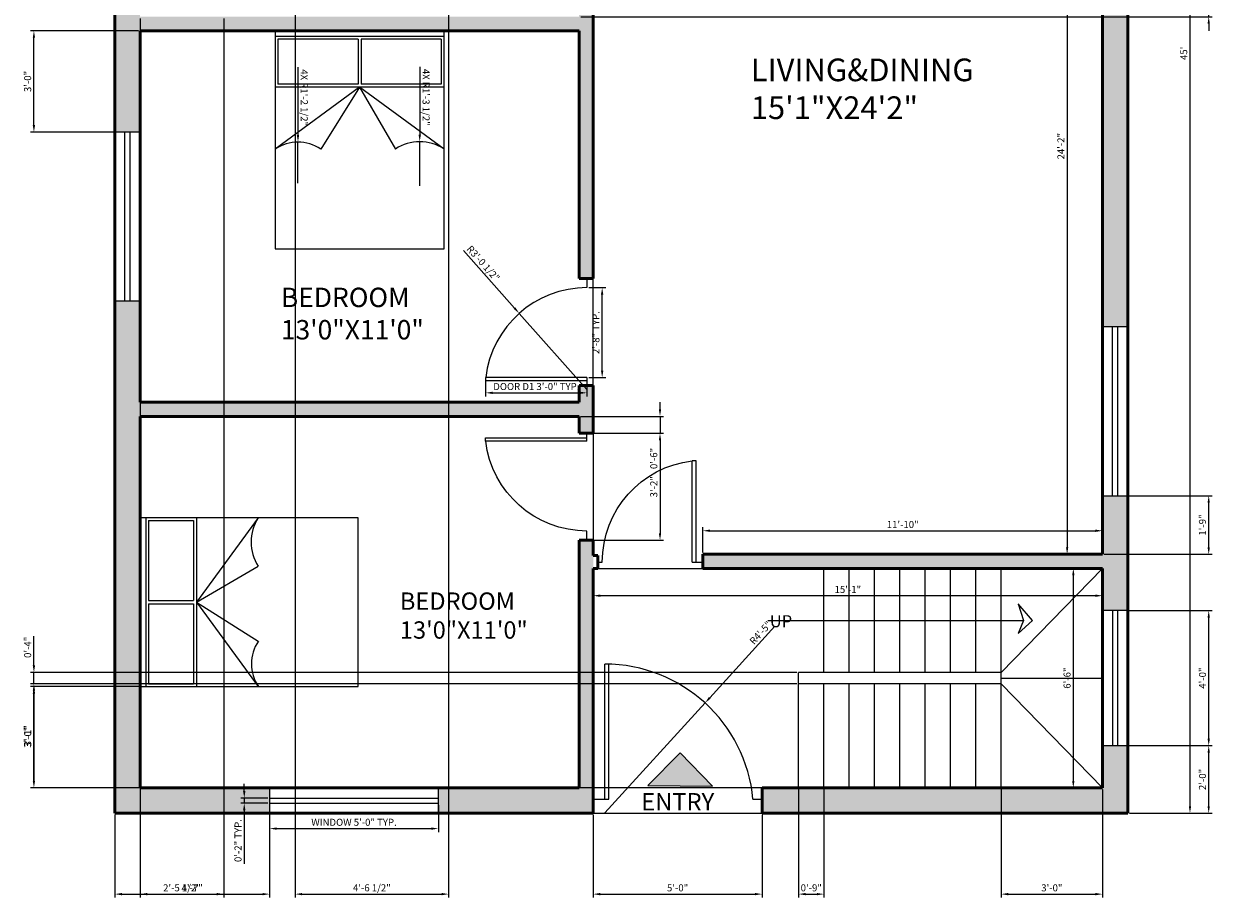
# Model space of a CAD drawing. Units: inches. Extents: x 457 to 882, y 0 to 1111.
# Tile 2 of 4: x 459 to 881, y 506 to 817. Entities that reach past the tile are written whole.
import ezdxf

# ---------------------------------------------------------------- set-up
doc = ezdxf.new("R2010")
doc.units = ezdxf.units.IN
for name, color, linetype, lineweight in [('A-ANNO-DIMS', 2, 'Continuous', 18), ('A-ANNO-SYMB', 7, 'Continuous', 18), ('A-ANNO-SYMB-PATT', 8, 'Continuous', 13), ('A-ANNO-TEXT', 7, 'Continuous', 18), ('A-AREA-IDEN', 7, 'Continuous', 25), ('A-DOOR', 3, 'Continuous', 25), ('A-DOOR-THRE', 8, 'Continuous', 13), ('A-FLOR-STRS', 7, 'Continuous', 25), ('A-FURN', 8, 'Continuous', 18), ('A-GLAZ', 5, 'Continuous', 18), ('A-WALL', 7, 'Continuous', 50), ('A-WALL-PATT', 252, 'Continuous', 13)]:
    doc.layers.add(name, color=color, linetype=linetype, lineweight=lineweight)
doc.styles.get("Standard").update_dxf_attribs({"font": 'arial.ttf'})
doc.dimstyles.new('ISO-25', dxfattribs={"dimtxt": 2.5, "dimasz": 2.5, "dimexe": 1.25, "dimexo": 0.625, "dimtad": 1, "dimdec": 0, "dimlunit": 3, "dimtxsty": 'Standard', "dimcen": 2.5, "dimadec": 0, "dimazin": 0, "dimtfac": 1, "dimtdec": 0, "dimtmove": 0, "dimatfit": 3, "dimfxl": 1, "dimarcsym": 0})

# ---------------------------------------------------------------- blocks, each defined once
blk = doc.blocks.new('*D1')
at = {"layer": 'A-ANNO-DIMS', "color": 0, "lineweight": -2, "transparency": 16777216}
for p, q in [((841.63, 623.51), (830.64, 623.51)), ((831.89, 621.01), (831.89, 548.01)), ((841.63, 545.51), (830.64, 545.51))]:
    blk.add_line(p, q, dxfattribs=at)
at = {"layer": 'A-ANNO-DIMS', "color": 0, "transparency": 16777216}
for points in [[(831.47, 621.01), (832.31, 621.01), (831.89, 623.51)], [(831.47, 548.01), (832.31, 548.01), (831.89, 545.51)]]:
    blk.add_solid(points, dxfattribs=at)
at = {"layer": 'Defpoints', "color": 0, "transparency": 16777216}
for p in [(842.26, 623.51), (831.89, 545.51), (842.26, 545.51)]:
    blk.add_point(p, dxfattribs=at)
at = {"layer": 'A-ANNO-DIMS', "color": 0, "transparency": 16777216, "insert": (829.99, 584.51), "char_height": 2.5, "attachment_point": 5, "rotation": 90}
blk.add_mtext('6\'-6"', dxfattribs=at)
blk = doc.blocks.new('*D3')
at = {"layer": 'A-ANNO-DIMS', "color": 0, "lineweight": -2, "transparency": 16777216}
for p, q in [((851.88, 1076.51), (874.6, 1076.51)), ((873.35, 1074.01), (873.35, 539.01)), ((851.88, 536.51), (874.6, 536.51))]:
    blk.add_line(p, q, dxfattribs=at)
at = {"layer": 'A-ANNO-DIMS', "color": 0, "transparency": 16777216}
for points in [[(872.93, 1074.01), (873.76, 1074.01), (873.35, 1076.51)], [(872.93, 539.01), (873.76, 539.01), (873.35, 536.51)]]:
    blk.add_solid(points, dxfattribs=at)
at = {"layer": 'Defpoints', "color": 0, "transparency": 16777216}
for p in [(851.26, 1076.51), (851.26, 536.51), (873.35, 536.51)]:
    blk.add_point(p, dxfattribs=at)
at = {"layer": 'A-ANNO-DIMS', "color": 0, "transparency": 16777216, "insert": (871.45, 806.51), "char_height": 2.5, "attachment_point": 5, "rotation": 90}
blk.add_mtext("45'", dxfattribs=at)
blk = doc.blocks.new('*D5')
at = {"layer": 'A-ANNO-DIMS', "color": 0, "lineweight": -2, "transparency": 16777216}
for p, q in [((700.26, 629.13), (700.26, 638.12)), ((842.26, 629.13), (842.26, 638.12)), ((702.76, 636.87), (839.76, 636.87))]:
    blk.add_line(p, q, dxfattribs=at)
at = {"layer": 'A-ANNO-DIMS', "color": 0, "transparency": 16777216}
for points in [[(702.76, 637.29), (702.76, 636.46), (700.26, 636.87)], [(839.76, 637.29), (839.76, 636.46), (842.26, 636.87)]]:
    blk.add_solid(points, dxfattribs=at)
at = {"layer": 'Defpoints', "color": 0, "transparency": 16777216}
for p in [(842.26, 636.87), (700.26, 628.51), (842.26, 628.51)]:
    blk.add_point(p, dxfattribs=at)
at = {"layer": 'A-ANNO-DIMS', "color": 0, "transparency": 16777216, "insert": (771.26, 638.77), "char_height": 2.5, "attachment_point": 5}
blk.add_mtext('11\'-10"', dxfattribs=at)
blk = doc.blocks.new('*D7')
at = {"layer": 'A-ANNO-DIMS', "color": 0, "lineweight": -2, "transparency": 16777216}
for p, q in [((841.63, 918.51), (828.45, 918.51)), ((829.7, 916.01), (829.7, 631.01)), ((841.63, 628.51), (828.45, 628.51))]:
    blk.add_line(p, q, dxfattribs=at)
at = {"layer": 'A-ANNO-DIMS', "color": 0, "transparency": 16777216}
for points in [[(829.28, 916.01), (830.11, 916.01), (829.7, 918.51)], [(829.28, 631.01), (830.11, 631.01), (829.7, 628.51)]]:
    blk.add_solid(points, dxfattribs=at)
at = {"layer": 'Defpoints', "color": 0, "transparency": 16777216}
for p in [(842.26, 918.51), (829.7, 628.51), (842.26, 628.51)]:
    blk.add_point(p, dxfattribs=at)
at = {"layer": 'A-ANNO-DIMS', "color": 0, "transparency": 16777216, "insert": (827.82, 773.51), "char_height": 2.5, "attachment_point": 5, "rotation": 90}
blk.add_mtext('24\'-2"', dxfattribs=at)
blk = doc.blocks.new('*D8')
at = {"layer": 'A-ANNO-DIMS', "color": 0, "lineweight": -2, "transparency": 16777216}
for p, q in [((661.26, 622.88), (661.26, 612.55)), ((842.26, 622.88), (842.26, 612.55)), ((839.76, 613.8), (663.76, 613.8))]:
    blk.add_line(p, q, dxfattribs=at)
at = {"layer": 'A-ANNO-DIMS', "color": 0, "transparency": 16777216}
for points in [[(663.76, 614.22), (663.76, 613.38), (661.26, 613.8)], [(839.76, 614.22), (839.76, 613.38), (842.26, 613.8)]]:
    blk.add_solid(points, dxfattribs=at)
at = {"layer": 'Defpoints', "color": 0, "transparency": 16777216}
for p in [(661.26, 623.51), (842.26, 623.51), (661.26, 613.8)]:
    blk.add_point(p, dxfattribs=at)
at = {"layer": 'A-ANNO-DIMS', "color": 0, "transparency": 16777216, "insert": (751.76, 615.7), "char_height": 2.5, "attachment_point": 5}
blk.add_mtext('15\'-1"', dxfattribs=at)
blk = doc.blocks.new('BED-DOUBLE-60')
for p, q in [((0, 77.49), (0, 0)), ((60, 77.49), (0, 77.49)), ((60, 0), (60, 77.49)), ((60, 75.49), (0, 75.49)), ((29.44, 74.49), (0.94, 74.49)), ((0.94, 74.49), (0.94, 58.49)), ((29.44, 74.49), (29.44, 58.49)), ((59, 74.49), (30.53, 74.49)), ((30.53, 74.49), (30.53, 58.49)), ((59, 74.49), (59, 58.49)), ((60, 57.49), (0, 57.49)), ((30, 57.49), (0, 35.49)), ((29.44, 58.49), (0.94, 58.49)), ((30, 57.49), (16.16, 35.49)), ((60, 35.49), (30, 57.49)), ((30, 57.49), (42.73, 35.49)), ((59, 58.49), (30.53, 58.49)), ((0, 0), (60, 0))]:
    blk.add_line(p, q)
for centre, radius, start, end in [((51.36, 22.4), 15.69, 56.5972, 123.4028), ((8.08, 23.34), 14.59, 56.3669, 123.6331)]:
    blk.add_arc(centre, radius, start, end)
blk = doc.blocks.new('WIN-60-GLAZING')
for p, q in [((0, 0), (0, 60)), ((1.86, 0), (1.86, 60))]:
    blk.add_line(p, q)
blk = doc.blocks.new('DOOR-36-SWING')
blk.add_line((36, 0), (0, 0))
blk.add_arc((36, -4.26), 36.25, 90, 173.2534)
blk = doc.blocks.new('*D14')
at = {"layer": 'A-ANNO-DIMS', "color": 0, "lineweight": -2, "transparency": 16777216}
for p, q in [((546.26, 539.41), (546.26, 529.79)), ((606.26, 539.41), (606.26, 529.79)), ((548.76, 531.04), (603.76, 531.04))]:
    blk.add_line(p, q, dxfattribs=at)
at = {"layer": 'A-ANNO-DIMS', "color": 0, "transparency": 16777216}
for points in [[(548.76, 531.45), (548.76, 530.62), (546.26, 531.04)], [(603.76, 531.45), (603.76, 530.62), (606.26, 531.04)]]:
    blk.add_solid(points, dxfattribs=at)
at = {"layer": 'Defpoints', "color": 0, "transparency": 16777216}
for p in [(546.26, 540.04), (606.26, 540.04), (606.26, 531.04)]:
    blk.add_point(p, dxfattribs=at)
at = {"layer": 'A-ANNO-DIMS', "color": 0, "transparency": 16777216, "insert": (576.26, 532.96), "char_height": 2.5, "attachment_point": 5}
blk.add_mtext('WINDOW 5\'-0" TYP.', dxfattribs=at)
blk = doc.blocks.new('*D15')
at = {"layer": 'A-ANNO-DIMS', "color": 0, "lineweight": -2, "transparency": 16777216}
for p, q in [((537.26, 544.4), (537.26, 546.9)), ((545.63, 541.9), (536.01, 541.9)), ((537.26, 541.9), (537.26, 540.04)), ((545.63, 540.04), (536.01, 540.04)), ((537.26, 537.54), (537.26, 518.55))]:
    blk.add_line(p, q, dxfattribs=at)
at = {"layer": 'A-ANNO-DIMS', "color": 0, "transparency": 16777216}
for points in [[(536.84, 544.4), (537.67, 544.4), (537.26, 541.9)], [(536.84, 537.54), (537.67, 537.54), (537.26, 540.04)]]:
    blk.add_solid(points, dxfattribs=at)
at = {"layer": 'Defpoints', "color": 0, "transparency": 16777216}
for p in [(546.26, 541.9), (537.26, 540.04), (546.26, 540.04)]:
    blk.add_point(p, dxfattribs=at)
at = {"layer": 'A-ANNO-DIMS', "color": 0, "transparency": 16777216, "insert": (535.36, 526.79), "char_height": 2.5, "attachment_point": 5, "rotation": 90}
blk.add_mtext('0\'-2" TYP.', dxfattribs=at)
blk = doc.blocks.new('*D18')
at = {"layer": 'A-ANNO-DIMS', "color": 0, "lineweight": -2, "transparency": 16777216}
for p, q in [((623.05, 690.65), (623.05, 684.62)), ((659.05, 690.65), (659.05, 684.62)), ((625.55, 685.87), (656.55, 685.87))]:
    blk.add_line(p, q, dxfattribs=at)
at = {"layer": 'A-ANNO-DIMS', "color": 0, "transparency": 16777216}
for points in [[(625.55, 686.29), (625.55, 685.46), (623.05, 685.87)], [(656.55, 686.29), (656.55, 685.46), (659.05, 685.87)]]:
    blk.add_solid(points, dxfattribs=at)
at = {"layer": 'Defpoints', "color": 0, "transparency": 16777216}
for p in [(623.05, 691.27), (659.05, 691.27), (659.05, 685.87)]:
    blk.add_point(p, dxfattribs=at)
at = {"layer": 'A-ANNO-DIMS', "color": 0, "transparency": 16777216, "insert": (641.05, 687.79), "char_height": 2.5, "attachment_point": 5}
blk.add_mtext('DOOR D1 3\'-0" TYP.', dxfattribs=at)
blk = doc.blocks.new('*D19')
at = {"layer": 'A-ANNO-DIMS', "color": 0, "lineweight": -2, "transparency": 16777216}
for p, q in [((659.68, 723.27), (665.7, 723.27)), ((664.45, 693.77), (664.45, 720.77)), ((659.68, 691.27), (665.7, 691.27))]:
    blk.add_line(p, q, dxfattribs=at)
at = {"layer": 'A-ANNO-DIMS', "color": 0, "transparency": 16777216}
for points in [[(664.03, 720.77), (664.87, 720.77), (664.45, 723.27)], [(664.03, 693.77), (664.87, 693.77), (664.45, 691.27)]]:
    blk.add_solid(points, dxfattribs=at)
at = {"layer": 'Defpoints', "color": 0, "transparency": 16777216}
for p in [(659.05, 723.27), (664.45, 723.27), (659.05, 691.27)]:
    blk.add_point(p, dxfattribs=at)
at = {"layer": 'A-ANNO-DIMS', "color": 0, "transparency": 16777216, "insert": (662.55, 707.27), "char_height": 2.5, "attachment_point": 5, "rotation": 90}
blk.add_mtext('2\'-8" TYP.', dxfattribs=at)
blk = doc.blocks.new('*D25')
at = {"layer": 'A-ANNO-DIMS', "color": 0, "lineweight": -2, "transparency": 16777216}
for p, q in [((656.88, 671.51), (686.26, 671.51)), ((685.01, 669.01), (685.01, 636.01)), ((656.88, 633.51), (686.26, 633.51))]:
    blk.add_line(p, q, dxfattribs=at)
at = {"layer": 'A-ANNO-DIMS', "color": 0, "transparency": 16777216}
for points in [[(684.59, 669.01), (685.42, 669.01), (685.01, 671.51)], [(684.59, 636.01), (685.42, 636.01), (685.01, 633.51)]]:
    blk.add_solid(points, dxfattribs=at)
at = {"layer": 'Defpoints', "color": 0, "transparency": 16777216}
for p in [(656.26, 671.51), (656.26, 633.51), (685.01, 633.51)]:
    blk.add_point(p, dxfattribs=at)
at = {"layer": 'A-ANNO-DIMS', "color": 0, "transparency": 16777216, "insert": (683.11, 652.51), "char_height": 2.5, "attachment_point": 5, "rotation": 90}
blk.add_mtext('3\'-2"', dxfattribs=at)
blk = doc.blocks.new('*D26')
at = {"layer": 'A-ANNO-DIMS', "color": 0, "lineweight": -2, "transparency": 16777216}
for p, q in [((685.01, 680.01), (685.01, 682.51)), ((656.88, 677.51), (686.26, 677.51)), ((685.01, 677.51), (685.01, 671.51)), ((656.88, 671.51), (686.26, 671.51)), ((685.01, 669.01), (685.01, 658.61))]:
    blk.add_line(p, q, dxfattribs=at)
at = {"layer": 'A-ANNO-DIMS', "color": 0, "transparency": 16777216}
for points in [[(684.59, 680.01), (685.42, 680.01), (685.01, 677.51)], [(684.59, 669.01), (685.42, 669.01), (685.01, 671.51)]]:
    blk.add_solid(points, dxfattribs=at)
at = {"layer": 'Defpoints', "color": 0, "transparency": 16777216}
for p in [(656.26, 677.51), (656.26, 671.51), (685.01, 671.51)]:
    blk.add_point(p, dxfattribs=at)
at = {"layer": 'A-ANNO-DIMS', "color": 0, "transparency": 16777216, "insert": (683.11, 662.56), "char_height": 2.5, "attachment_point": 5, "rotation": 90}
blk.add_mtext('0\'-6"', dxfattribs=at)
blk = doc.blocks.new('*D32')
at = {"layer": 'A-ANNO-DIMS', "color": 0, "lineweight": -2, "transparency": 16777216}
for p, q in [((499.63, 814.51), (461.26, 814.51)), ((462.51, 781.01), (462.51, 812.01)), ((490.63, 778.51), (461.26, 778.51))]:
    blk.add_line(p, q, dxfattribs=at)
at = {"layer": 'A-ANNO-DIMS', "color": 0, "transparency": 16777216}
for points in [[(462.09, 812.01), (462.92, 812.01), (462.51, 814.51)], [(462.09, 781.01), (462.92, 781.01), (462.51, 778.51)]]:
    blk.add_solid(points, dxfattribs=at)
at = {"layer": 'Defpoints', "color": 0, "transparency": 16777216}
for p in [(462.51, 814.51), (500.26, 814.51), (491.26, 778.51)]:
    blk.add_point(p, dxfattribs=at)
at = {"layer": 'A-ANNO-DIMS', "color": 0, "transparency": 16777216, "insert": (460.61, 796.51), "char_height": 2.5, "attachment_point": 5, "rotation": 90}
blk.add_mtext('3\'-0"', dxfattribs=at)
blk = doc.blocks.new('*D33')
at = {"layer": 'A-ANNO-DIMS', "color": 0, "lineweight": -2, "transparency": 16777216}
for p, q in [((491.26, 535.88), (491.26, 506.51)), ((546.26, 535.88), (546.26, 506.51)), ((493.76, 507.76), (543.76, 507.76))]:
    blk.add_line(p, q, dxfattribs=at)
at = {"layer": 'A-ANNO-DIMS', "color": 0, "transparency": 16777216}
for points in [[(493.76, 508.17), (493.76, 507.34), (491.26, 507.76)], [(543.76, 508.17), (543.76, 507.34), (546.26, 507.76)]]:
    blk.add_solid(points, dxfattribs=at)
at = {"layer": 'Defpoints', "color": 0, "transparency": 16777216}
for p in [(491.26, 536.51), (546.26, 536.51), (546.26, 507.76)]:
    blk.add_point(p, dxfattribs=at)
at = {"layer": 'A-ANNO-DIMS', "color": 0, "transparency": 16777216, "insert": (518.76, 509.63), "char_height": 2.5, "attachment_point": 5}
blk.add_mtext('4\'-7"', dxfattribs=at)
blk = doc.blocks.new('*D35')
at = {"layer": 'A-ANNO-DIMS', "color": 0, "lineweight": -2, "transparency": 16777216}
for p, q in [((851.88, 649.3), (881.26, 649.3)), ((880.01, 631.01), (880.01, 646.8)), ((842.88, 628.51), (881.26, 628.51))]:
    blk.add_line(p, q, dxfattribs=at)
at = {"layer": 'A-ANNO-DIMS', "color": 0, "transparency": 16777216}
for points in [[(879.59, 646.8), (880.42, 646.8), (880.01, 649.3)], [(879.59, 631.01), (880.42, 631.01), (880.01, 628.51)]]:
    blk.add_solid(points, dxfattribs=at)
at = {"layer": 'Defpoints', "color": 0, "transparency": 16777216}
for p in [(851.26, 649.3), (880.01, 649.3), (842.26, 628.51)]:
    blk.add_point(p, dxfattribs=at)
at = {"layer": 'A-ANNO-DIMS', "color": 0, "transparency": 16777216, "insert": (878.11, 638.9), "char_height": 2.5, "attachment_point": 5, "rotation": 90}
blk.add_mtext('1\'-9"', dxfattribs=at)
blk = doc.blocks.new('*D38')
at = {"layer": 'A-ANNO-DIMS', "color": 0, "lineweight": -2, "transparency": 16777216}
for p, q in [((851.88, 608.51), (881.26, 608.51)), ((880.01, 563.01), (880.01, 606.01)), ((851.88, 560.51), (881.26, 560.51))]:
    blk.add_line(p, q, dxfattribs=at)
at = {"layer": 'A-ANNO-DIMS', "color": 0, "transparency": 16777216}
for points in [[(879.59, 606.01), (880.42, 606.01), (880.01, 608.51)], [(879.59, 563.01), (880.42, 563.01), (880.01, 560.51)]]:
    blk.add_solid(points, dxfattribs=at)
at = {"layer": 'Defpoints', "color": 0, "transparency": 16777216}
for p in [(851.26, 608.51), (880.01, 608.51), (851.26, 560.51)]:
    blk.add_point(p, dxfattribs=at)
at = {"layer": 'A-ANNO-DIMS', "color": 0, "transparency": 16777216, "insert": (878.11, 584.51), "char_height": 2.5, "attachment_point": 5, "rotation": 90}
blk.add_mtext('4\'-0"', dxfattribs=at)
blk = doc.blocks.new('*D39')
at = {"layer": 'A-ANNO-DIMS', "color": 0, "lineweight": -2, "transparency": 16777216}
for p, q in [((851.88, 560.51), (881.26, 560.51)), ((880.01, 539.01), (880.01, 558.01)), ((851.88, 536.51), (881.26, 536.51))]:
    blk.add_line(p, q, dxfattribs=at)
at = {"layer": 'A-ANNO-DIMS', "color": 0, "transparency": 16777216}
for points in [[(879.59, 558.01), (880.42, 558.01), (880.01, 560.51)], [(879.59, 539.01), (880.42, 539.01), (880.01, 536.51)]]:
    blk.add_solid(points, dxfattribs=at)
at = {"layer": 'Defpoints', "color": 0, "transparency": 16777216}
for p in [(851.26, 560.51), (880.01, 560.51), (851.26, 536.51)]:
    blk.add_point(p, dxfattribs=at)
at = {"layer": 'A-ANNO-DIMS', "color": 0, "transparency": 16777216, "insert": (878.11, 548.51), "char_height": 2.5, "attachment_point": 5, "rotation": 90}
blk.add_mtext('2\'-0"', dxfattribs=at)
blk = doc.blocks.new('*D40')
at = {"layer": 'A-ANNO-DIMS', "color": 0, "lineweight": -2, "transparency": 16777216}
for p, q in [((661.26, 535.88), (661.26, 506.51)), ((721.26, 535.88), (721.26, 506.51)), ((663.76, 507.76), (718.76, 507.76))]:
    blk.add_line(p, q, dxfattribs=at)
at = {"layer": 'A-ANNO-DIMS', "color": 0, "transparency": 16777216}
for points in [[(663.76, 508.17), (663.76, 507.34), (661.26, 507.76)], [(718.76, 508.17), (718.76, 507.34), (721.26, 507.76)]]:
    blk.add_solid(points, dxfattribs=at)
at = {"layer": 'Defpoints', "color": 0, "transparency": 16777216}
for p in [(661.26, 536.51), (721.26, 536.51), (721.26, 507.76)]:
    blk.add_point(p, dxfattribs=at)
at = {"layer": 'A-ANNO-DIMS', "color": 0, "transparency": 16777216, "insert": (691.26, 509.66), "char_height": 2.5, "attachment_point": 5}
blk.add_mtext('5\'-0"', dxfattribs=at)
blk = doc.blocks.new('*D41')
at = {"layer": 'A-ANNO-DIMS', "color": 0, "lineweight": -2, "transparency": 16777216}
for p, q in [((734.26, 544.88), (734.26, 506.51)), ((743.26, 544.88), (743.26, 506.51)), ((736.76, 507.76), (740.76, 507.76))]:
    blk.add_line(p, q, dxfattribs=at)
at = {"layer": 'A-ANNO-DIMS', "color": 0, "transparency": 16777216}
for points in [[(736.76, 508.17), (736.76, 507.34), (734.26, 507.76)], [(740.76, 508.17), (740.76, 507.34), (743.26, 507.76)]]:
    blk.add_solid(points, dxfattribs=at)
at = {"layer": 'Defpoints', "color": 0, "transparency": 16777216}
for p in [(734.26, 545.51), (743.26, 545.51), (743.26, 507.76)]:
    blk.add_point(p, dxfattribs=at)
at = {"layer": 'A-ANNO-DIMS', "color": 0, "transparency": 16777216, "insert": (738.76, 509.66), "char_height": 2.5, "attachment_point": 5}
blk.add_mtext('0\'-9"', dxfattribs=at)
blk = doc.blocks.new('*D42')
at = {"layer": 'A-ANNO-DIMS', "color": 0, "lineweight": -2, "transparency": 16777216}
for p, q in [((806.26, 544.88), (806.26, 506.51)), ((842.26, 544.88), (842.26, 506.51)), ((808.76, 507.76), (839.76, 507.76))]:
    blk.add_line(p, q, dxfattribs=at)
at = {"layer": 'A-ANNO-DIMS', "color": 0, "transparency": 16777216}
for points in [[(808.76, 508.17), (808.76, 507.34), (806.26, 507.76)], [(839.76, 508.17), (839.76, 507.34), (842.26, 507.76)]]:
    blk.add_solid(points, dxfattribs=at)
at = {"layer": 'Defpoints', "color": 0, "transparency": 16777216}
for p in [(806.26, 545.51), (842.26, 545.51), (842.26, 507.76)]:
    blk.add_point(p, dxfattribs=at)
at = {"layer": 'A-ANNO-DIMS', "color": 0, "transparency": 16777216, "insert": (824.26, 509.66), "char_height": 2.5, "attachment_point": 5}
blk.add_mtext('3\'-0"', dxfattribs=at)
blk = doc.blocks.new('*D43')
at = {"layer": 'A-ANNO-DIMS', "color": 0, "lineweight": -2, "transparency": 16777216}
for p, q in [((733.63, 582.51), (461.26, 582.51)), ((462.51, 548.01), (462.51, 580.01)), ((733.63, 545.51), (461.26, 545.51))]:
    blk.add_line(p, q, dxfattribs=at)
at = {"layer": 'A-ANNO-DIMS', "color": 0, "transparency": 16777216}
for points in [[(462.09, 580.01), (462.92, 580.01), (462.51, 582.51)], [(462.09, 548.01), (462.92, 548.01), (462.51, 545.51)]]:
    blk.add_solid(points, dxfattribs=at)
at = {"layer": 'Defpoints', "color": 0, "transparency": 16777216}
for p in [(462.51, 582.51), (734.26, 582.51), (734.26, 545.51)]:
    blk.add_point(p, dxfattribs=at)
at = {"layer": 'A-ANNO-DIMS', "color": 0, "transparency": 16777216, "insert": (460.61, 564.01), "char_height": 2.5, "attachment_point": 5, "rotation": 90}
blk.add_mtext('3\'-1"', dxfattribs=at)
blk = doc.blocks.new('*D44')
at = {"layer": 'A-ANNO-DIMS', "color": 0, "lineweight": -2, "transparency": 16777216}
for p, q in [((462.51, 589.01), (462.51, 599.4)), ((733.63, 586.51), (461.26, 586.51)), ((462.51, 582.51), (462.51, 586.51)), ((733.63, 582.51), (461.26, 582.51)), ((462.51, 580.01), (462.51, 577.51))]:
    blk.add_line(p, q, dxfattribs=at)
at = {"layer": 'A-ANNO-DIMS', "color": 0, "transparency": 16777216}
for points in [[(462.09, 589.01), (462.92, 589.01), (462.51, 586.51)], [(462.09, 580.01), (462.92, 580.01), (462.51, 582.51)]]:
    blk.add_solid(points, dxfattribs=at)
at = {"layer": 'Defpoints', "color": 0, "transparency": 16777216}
for p in [(462.51, 586.51), (734.26, 586.51), (734.26, 582.51)]:
    blk.add_point(p, dxfattribs=at)
at = {"layer": 'A-ANNO-DIMS', "color": 0, "transparency": 16777216, "insert": (460.61, 595.45), "char_height": 2.5, "attachment_point": 5, "rotation": 90}
blk.add_mtext('0\'-4"', dxfattribs=at)
blk = doc.blocks.new('*D45')
at = {"layer": 'A-ANNO-DIMS', "color": 0, "lineweight": -2, "transparency": 16777216}
for p, q in [((500.26, 818.88), (500.26, 506.51)), ((530, 818.88), (530, 506.51)), ((502.76, 507.76), (527.5, 507.76))]:
    blk.add_line(p, q, dxfattribs=at)
at = {"layer": 'A-ANNO-DIMS', "color": 0, "transparency": 16777216}
for points in [[(502.76, 508.17), (502.76, 507.34), (500.26, 507.76)], [(527.5, 508.17), (527.5, 507.34), (530, 507.76)]]:
    blk.add_solid(points, dxfattribs=at)
at = {"layer": 'Defpoints', "color": 0, "transparency": 16777216}
for p in [(500.26, 819.51), (530, 819.51), (530, 507.76)]:
    blk.add_point(p, dxfattribs=at)
at = {"layer": 'A-ANNO-DIMS', "color": 0, "transparency": 16777216, "insert": (515.13, 509.67), "char_height": 2.5, "attachment_point": 5}
blk.add_mtext('2\'-5 1/2"', dxfattribs=at)
blk = doc.blocks.new('*D48')
at = {"layer": 'A-ANNO-DIMS', "color": 0, "lineweight": -2, "transparency": 16777216}
for p, q in [((880.01, 828.01), (880.01, 838.4)), ((656.88, 825.51), (881.26, 825.51)), ((880.01, 819.51), (880.01, 825.51)), ((656.88, 819.51), (881.26, 819.51)), ((880.01, 817.01), (880.01, 814.51))]:
    blk.add_line(p, q, dxfattribs=at)
at = {"layer": 'A-ANNO-DIMS', "color": 0, "transparency": 16777216}
for points in [[(879.59, 828.01), (880.42, 828.01), (880.01, 825.51)], [(879.59, 817.01), (880.42, 817.01), (880.01, 819.51)]]:
    blk.add_solid(points, dxfattribs=at)
at = {"layer": 'Defpoints', "color": 0, "transparency": 16777216}
for p in [(656.26, 825.51), (880.01, 825.51), (656.26, 819.51)]:
    blk.add_point(p, dxfattribs=at)
at = {"layer": 'A-ANNO-DIMS', "color": 0, "transparency": 16777216, "insert": (878.11, 834.45), "char_height": 2.5, "attachment_point": 5, "rotation": 90}
blk.add_mtext('0\'-6"', dxfattribs=at)
blk = doc.blocks.new('*D56')
at = {"layer": 'A-ANNO-DIMS', "color": 0, "lineweight": -2, "transparency": 16777216}
for p, q in [((555.33, 898.14), (555.33, 506.51)), ((609.9, 898.14), (609.9, 506.51)), ((557.83, 507.76), (607.4, 507.76))]:
    blk.add_line(p, q, dxfattribs=at)
at = {"layer": 'A-ANNO-DIMS', "color": 0, "transparency": 16777216}
for points in [[(557.83, 508.17), (557.83, 507.34), (555.33, 507.76)], [(607.4, 508.17), (607.4, 507.34), (609.9, 507.76)]]:
    blk.add_solid(points, dxfattribs=at)
at = {"layer": 'Defpoints', "color": 0, "transparency": 16777216}
for p in [(555.33, 898.77), (609.9, 898.77), (609.9, 507.76)]:
    blk.add_point(p, dxfattribs=at)
at = {"layer": 'A-ANNO-DIMS', "color": 0, "transparency": 16777216, "insert": (582.61, 509.67), "char_height": 2.5, "attachment_point": 5}
blk.add_mtext('4\'-6 1/2"', dxfattribs=at)
blk = doc.blocks.new('*D60')
at = {"layer": 'A-ANNO-DIMS', "color": 0, "lineweight": -2, "transparency": 16777216}
for p, q in [((499.63, 581.51), (461.26, 581.51)), ((462.51, 579.01), (462.51, 548.01)), ((499.63, 545.51), (461.26, 545.51))]:
    blk.add_line(p, q, dxfattribs=at)
at = {"layer": 'A-ANNO-DIMS', "color": 0, "transparency": 16777216}
for points in [[(462.09, 579.01), (462.92, 579.01), (462.51, 581.51)], [(462.09, 548.01), (462.92, 548.01), (462.51, 545.51)]]:
    blk.add_solid(points, dxfattribs=at)
at = {"layer": 'Defpoints', "color": 0, "transparency": 16777216}
for p in [(500.26, 581.51), (462.51, 545.51), (500.26, 545.51)]:
    blk.add_point(p, dxfattribs=at)
at = {"layer": 'A-ANNO-DIMS', "color": 0, "transparency": 16777216, "insert": (460.61, 563.51), "char_height": 2.5, "attachment_point": 5, "rotation": 90}
blk.add_mtext('3\'-0"', dxfattribs=at)
blk = doc.blocks.new('*D61')
at = {"layer": 'A-ANNO-DIMS', "color": 0, "lineweight": -2, "transparency": 16777216}
for p, q in [((725.86, 602.94), (702.7, 577.53)), ((665.39, 536.59), (701.01, 575.68))]:
    blk.add_line(p, q, dxfattribs=at)
at = {"layer": 'A-ANNO-DIMS', "color": 0, "transparency": 16777216}
blk.add_solid([(702.39, 577.81), (703.01, 577.25), (701.01, 575.68)], dxfattribs=at)
at = {"layer": 'Defpoints', "color": 0, "transparency": 16777216}
for p in [(701.01, 575.68), (665.39, 536.59)]:
    blk.add_point(p, dxfattribs=at)
at = {"layer": 'A-ANNO-DIMS', "color": 0, "transparency": 16777216, "insert": (720.99, 600.41), "char_height": 2.5, "attachment_point": 5, "rotation": 47.6519}
blk.add_mtext('R4\'-5"', dxfattribs=at)
blk = doc.blocks.new('*D68')
at = {"layer": 'A-ANNO-DIMS', "color": 0, "lineweight": -2, "transparency": 16777216}
for p, q in [((615.17, 736.39), (633.31, 715.98)), ((659.05, 687.01), (634.97, 714.11))]:
    blk.add_line(p, q, dxfattribs=at)
at = {"layer": 'A-ANNO-DIMS', "color": 0, "transparency": 16777216}
blk.add_solid([(633.62, 716.26), (633, 715.7), (634.97, 714.11)], dxfattribs=at)
at = {"layer": 'Defpoints', "color": 0, "transparency": 16777216}
for p in [(634.97, 714.11), (659.05, 687.01)]:
    blk.add_point(p, dxfattribs=at)
at = {"layer": 'A-ANNO-DIMS', "color": 0, "transparency": 16777216, "insert": (621.96, 731.64), "char_height": 2.5, "attachment_point": 5, "rotation": 311.6258}
blk.add_mtext('R3\'-0 1/2"', dxfattribs=at)
blk = doc.blocks.new('*D69')
at = {"layer": 'A-ANNO-DIMS', "color": 0, "lineweight": -2, "transparency": 16777216}
for p, q in [((599.62, 801.68), (599.62, 777.6)), ((599.62, 759.41), (599.62, 775.1))]:
    blk.add_line(p, q, dxfattribs=at)
at = {"layer": 'A-ANNO-DIMS', "color": 0, "transparency": 16777216}
blk.add_solid([(600.04, 777.6), (599.2, 777.6), (599.62, 775.1)], dxfattribs=at)
at = {"layer": 'Defpoints', "color": 0, "transparency": 16777216}
for p in [(599.62, 775.1), (599.62, 759.41)]:
    blk.add_point(p, dxfattribs=at)
at = {"layer": 'A-ANNO-DIMS', "color": 0, "transparency": 16777216, "insert": (601.54, 790.89), "char_height": 2.5, "attachment_point": 5, "rotation": 270.0015}
blk.add_mtext('4X R1\'-3 1/2"', dxfattribs=at)
blk = doc.blocks.new('*D70')
at = {"layer": 'A-ANNO-DIMS', "color": 0, "lineweight": -2, "transparency": 16777216}
for p, q in [((556.34, 801.53), (556.34, 777.45)), ((556.34, 760.35), (556.34, 774.95))]:
    blk.add_line(p, q, dxfattribs=at)
at = {"layer": 'A-ANNO-DIMS', "color": 0, "transparency": 16777216}
blk.add_solid([(556.76, 777.45), (555.92, 777.45), (556.34, 774.95)], dxfattribs=at)
at = {"layer": 'Defpoints', "color": 0, "transparency": 16777216}
for p in [(556.34, 774.95), (556.34, 760.35)]:
    blk.add_point(p, dxfattribs=at)
at = {"layer": 'A-ANNO-DIMS', "color": 0, "transparency": 16777216, "insert": (558.26, 790.74), "char_height": 2.5, "attachment_point": 5, "rotation": 270.001}
blk.add_mtext('4X R1\'-2 1/2"', dxfattribs=at)

msp = doc.modelspace()

# ---------------------------------------------------------------- hatches: boundary and pattern name
at = {"layer": 'A-ANNO-SYMB-PATT'}
h = msp.add_hatch(color=256, dxfattribs=at)
h.dxf.hatch_style = 1
h.paths.add_polyline_path([(692.14, 557.94), (680.67, 546.33), (703.61, 546.11)])
at = {"layer": 'A-WALL-PATT'}
h = msp.add_hatch(color=256, dxfattribs=at)
h.dxf.hatch_style = 1
h.paths.add_polyline_path([(677.26, 1076.51), (491.26, 1076.51), (491.26, 1031.73), (500.26, 1031.73), (500.26, 1067.51), (656.26, 1067.51), (656.26, 962.63), (661.26, 962.63), (661.26, 1067.51), (677.26, 1067.51)])
h.paths.add_polyline_path([(851.26, 1076.51), (701.26, 1076.51), (701.26, 1067.51), (717.26, 1067.51), (717.26, 971.51), (691.26, 971.51), (691.26, 966.51), (717.26, 966.51), (717.26, 962.63), (722.26, 962.63), (722.26, 1067.51), (842.26, 1067.51), (842.26, 1031.73), (851.26, 1031.73)])
h.paths.add_polyline_path([(851.26, 971.73), (842.26, 971.73), (842.26, 923.51), (722.26, 923.51), (722.26, 926.63), (717.26, 926.63), (717.26, 918.51), (842.26, 918.51), (842.26, 896.98), (851.26, 896.98)])
h.paths.add_polyline_path([(661.26, 926.63), (656.26, 926.63), (656.26, 923.51), (500.26, 923.51), (500.26, 971.73), (491.26, 971.73), (491.26, 899.01), (500.26, 899.01), (500.26, 918.51), (656.26, 918.51), (656.26, 873.51), (661.26, 873.51)])
h.paths.add_polyline_path([(500.26, 839.01), (491.26, 839.01), (491.26, 778.51), (500.26, 778.51), (500.26, 814.51), (656.26, 814.51), (656.26, 726.51), (661.26, 726.51), (661.26, 825.51), (656.26, 825.51), (656.26, 819.51), (500.26, 819.51)])
h.paths.add_polyline_path([(661.26, 633.51), (656.26, 633.51), (656.26, 545.51), (606.26, 545.51), (606.26, 536.51), (661.26, 536.51)], flags=0)
h.paths.add_polyline_path([(851.26, 560.51), (842.26, 560.51), (842.26, 545.51), (721.26, 545.51), (721.26, 536.51), (851.26, 536.51)])
h.paths.add_polyline_path([(851.26, 649.3), (842.26, 649.3), (842.26, 628.51), (700.26, 628.51), (700.26, 623.51), (842.26, 623.51), (842.26, 608.51), (851.26, 608.51)])
h.paths.add_polyline_path([(500.26, 677.51), (656.26, 677.51), (656.26, 671.51), (661.26, 671.51), (661.26, 688.51), (656.26, 688.51), (656.26, 682.51), (500.26, 682.51), (500.26, 718.51), (491.26, 718.51), (491.26, 536.51), (546.26, 536.51), (546.26, 545.51), (500.26, 545.51)])
h = msp.add_hatch(color=256, dxfattribs=at)
h.dxf.hatch_style = 1
h.paths.add_polyline_path([(851.26, 836.98), (842.26, 836.98), (842.26, 709.3), (851.26, 709.3)])
h = msp.add_hatch(color=256, dxfattribs=at)
h.dxf.hatch_style = 1
h.paths.add_polyline_path([(661.26, 633.51), (656.26, 633.51), (656.26, 545.51), (606.26, 545.51), (606.26, 536.51), (661.26, 536.51)])

# ---------------------------------------------------------------- linework, layer by layer
at = {"layer": 'A-ANNO-SYMB'}
for p, q in [((817.38, 605.01), (812.27, 610.9)), ((812.27, 610.9), (814.15, 605.01)), ((723.36, 605.01), (814.15, 605.01)), ((812.27, 600.4), (817.38, 605.01)), ((814.15, 605.01), (812.27, 600.4)), ((692.14, 557.94), (680.67, 546.33)), ((703.61, 546.11), (692.14, 557.94)), ((680.67, 546.33), (703.61, 546.11))]:
    msp.add_line(p, q, dxfattribs=at)
at = {"layer": 'A-DOOR'}
for p, q in [((659.05, 726.51), (659.05, 723.27)), ((623.05, 691.27), (623.05, 690.24)), ((623.05, 690.24), (659.05, 690.24)), ((659.05, 691.27), (659.05, 688.51)), ((623.05, 668.74), (623.05, 669.86)), ((623.05, 669.86), (659.05, 669.86)), ((659.05, 668.74), (659.05, 671.51)), ((697.87, 661.73), (696.49, 661.73)), ((697.87, 625.73), (697.87, 661.73)), ((659.05, 633.51), (659.05, 636.74)), ((662.88, 625.73), (664.5, 625.73)), ((696.49, 625.73), (700.26, 625.73)), ((665.39, 541.48), (665.39, 589.48)), ((666.88, 541.48), (666.88, 589.48)), ((661.26, 541.48), (666.88, 541.48)), ((718.05, 541.48), (721.26, 541.48))]:
    msp.add_line(p, q, dxfattribs=at)
msp.add_arc((665.39, 536.59), 52.89, 5.3049, 90, dxfattribs=at)
at = {"layer": 'A-DOOR-THRE'}
for p, q in [((661.26, 688.51), (661.26, 726.51)), ((661.26, 671.51), (661.26, 633.51)), ((662.88, 623.51), (700.26, 623.51)), ((661.26, 536.51), (721.26, 536.51))]:
    msp.add_line(p, q, dxfattribs=at)
at = {"layer": 'A-FLOR-STRS'}
for p, q in [((743.26, 586.51), (743.26, 623.51)), ((752.26, 586.51), (752.26, 623.51)), ((761.26, 586.51), (761.26, 623.51)), ((770.26, 586.51), (770.26, 623.51)), ((779.26, 586.51), (779.26, 623.51)), ((788.26, 586.51), (788.26, 623.51)), ((797.26, 586.51), (797.26, 623.51)), ((806.26, 545.51), (806.26, 623.51)), ((806.26, 586.51), (842.26, 623.51)), ((806.26, 586.51), (734.26, 586.51)), ((734.26, 545.51), (734.26, 586.51)), ((806.26, 584.51), (842.26, 584.51)), ((806.26, 582.51), (734.26, 582.51)), ((743.26, 545.51), (743.26, 582.51)), ((752.26, 545.51), (752.26, 582.51)), ((761.26, 545.51), (761.26, 582.51)), ((770.26, 545.51), (770.26, 582.51)), ((779.26, 545.51), (779.26, 582.51)), ((788.26, 545.51), (788.26, 582.51)), ((797.26, 545.51), (797.26, 582.51)), ((806.26, 582.51), (842.26, 545.51))]:
    msp.add_line(p, q, dxfattribs=at)
at = {"layer": 'A-GLAZ'}
for p, q in [((500.26, 778.51), (491.26, 778.51)), ((491.26, 718.51), (500.26, 718.51)), ((851.26, 709.3), (842.26, 709.3)), ((842.26, 649.3), (851.26, 649.3)), ((851.26, 608.51), (842.26, 608.51)), ((845.79, 608.51), (845.79, 560.51)), ((847.65, 608.51), (847.65, 560.51)), ((842.26, 560.51), (851.26, 560.51)), ((546.26, 545.51), (546.26, 536.51)), ((606.26, 536.51), (606.26, 545.51))]:
    msp.add_line(p, q, dxfattribs=at)
at = {"layer": 'A-WALL'}
for p, q in [((491.26, 1076.51), (491.26, 536.51)), ((851.26, 536.51), (851.26, 1076.51)), ((842.26, 628.51), (842.26, 918.51)), ((661.26, 825.51), (661.26, 726.51)), ((500.26, 814.51), (656.26, 814.51)), ((500.26, 814.51), (500.26, 682.51)), ((656.26, 814.51), (656.26, 726.51)), ((661.26, 726.51), (656.26, 726.51)), ((661.26, 688.51), (656.26, 688.51)), ((656.26, 688.51), (656.26, 682.51)), ((661.26, 688.51), (661.26, 671.51)), ((500.26, 682.51), (656.26, 682.51)), ((500.26, 677.51), (656.26, 677.51)), ((500.26, 677.51), (500.26, 545.51)), ((656.26, 677.51), (656.26, 671.51)), ((661.26, 671.51), (656.26, 671.51)), ((661.26, 633.51), (656.26, 633.51)), ((656.26, 633.51), (656.26, 545.51)), ((661.26, 633.51), (661.26, 628.11)), ((662.88, 628.11), (661.26, 628.11)), ((662.88, 623.51), (662.88, 628.11)), ((662.88, 625.73), (662.88, 623.51)), ((700.26, 623.51), (700.26, 628.51)), ((700.26, 628.51), (842.26, 628.51)), ((662.88, 623.51), (661.26, 623.51)), ((661.26, 623.51), (661.26, 536.51)), ((700.26, 623.51), (842.26, 623.51)), ((842.26, 545.51), (842.26, 623.51)), ((500.26, 545.51), (656.26, 545.51)), ((721.26, 536.51), (721.26, 545.51)), ((721.26, 545.51), (842.26, 545.51)), ((491.26, 536.51), (661.26, 536.51)), ((721.26, 536.51), (851.26, 536.51))]:
    msp.add_line(p, q, dxfattribs=at)

# ---------------------------------------------------------------- block references
at = {"layer": 'A-DOOR'}
msp.add_blockref('DOOR-36-SWING', (623.05, 691.27), dxfattribs=at)
at = {"layer": 'A-DOOR', "extrusion": (0, 0, -1), "zscale": -1}
for p, rotation in [((-623.05, 668.74), 180), ((-696.49, 661.73), 269.9999999999999)]:
    msp.add_blockref('DOOR-36-SWING', p, dxfattribs=dict(at, rotation=rotation))
at = {"layer": 'A-FURN'}
msp.add_blockref('BED-DOUBLE-60', (548.26, 737.01), dxfattribs=at)
at = {"layer": 'A-FURN', "rotation": 90}
msp.add_blockref('BED-DOUBLE-60', (577.75, 581.51), dxfattribs=at)
at = {"layer": 'A-GLAZ'}
for p in [(494.86, 718.5), (845.86, 649.3)]:
    msp.add_blockref('WIN-60-GLAZING', p, dxfattribs=at)
at = {"layer": 'A-GLAZ', "rotation": 270.0000000000001}
msp.add_blockref('WIN-60-GLAZING', (546.26, 541.9), dxfattribs=at)

# ---------------------------------------------------------------- texts
at = {"layer": 'A-ANNO-TEXT', "attachment_point": 1}
for s, width, gutter_width, insert, char_height in [('UP', 56.9254, 21.47, (724.03, 606.87), 4.294), ('ENTRY', 81.9788, 30.92, (678.32, 543.67), 6.184)]:
    msp.add_mtext_dynamic_manual_height_columns(s, width=width, gutter_width=gutter_width, heights=[0], dxfattribs=dict(at, insert=insert, char_height=char_height))
at = {"layer": 'A-AREA-IDEN', "attachment_point": 1}
for s, width, gutter_width, insert, char_height in [('LIVING&DINING\\P15\'1"X24\'2"', 140.6069, 40.29, (717.27, 804.65), 8.058), ('BEDROOM\\P13\'0"X11\'0"', 91.3786, 34.46, (550.26, 723.23), 6.8929), ('BEDROOM\\P13\'0"X11\'0"', 78.4895, 30.8, (592.56, 614.95), 6.1598)]:
    msp.add_mtext_dynamic_manual_height_columns(s, width=width, gutter_width=gutter_width, heights=[0], dxfattribs=dict(at, insert=insert, char_height=char_height))

# ---------------------------------------------------------------- dimensions: what is measured, and where the dimension line sits
at = {"layer": 'A-ANNO-DIMS'}
for base, p1, p2, angle, override, picture, middle in [((873.35, 536.51), (851.26, 1076.51), (851.26, 536.51), 90, {"dimclrd": 0, "dimclre": 0, "dimclrt": 0}, '*D3', (871.45, 806.51)), ((829.7, 628.51), (842.26, 918.51), (842.26, 628.51), 90, {"dimclrd": 0, "dimclre": 0, "dimclrt": 0}, '*D7', (827.82, 773.51)), ((880.01, 825.51), (656.26, 819.51), (656.26, 825.51), 90, {"dimdec": 1, "dimlfac": 1, "dimrnd": 0, "dimzin": 1, "dimdsep": 46, "dimlunit": 4, "dimfrac": 2}, '*D48', (878.11, 834.45)), ((462.51, 814.51), (491.26, 778.51), (500.26, 814.51), 90, {"dimdec": 1, "dimlfac": 1, "dimrnd": 0, "dimzin": 1, "dimdsep": 46, "dimlunit": 4, "dimfrac": 2}, '*D32', (460.61, 796.51)), ((685.01, 671.51), (656.26, 677.51), (656.26, 671.51), 270, {"dimdec": 1, "dimlfac": 1, "dimrnd": 0, "dimzin": 1, "dimdsep": 46, "dimlunit": 4, "dimfrac": 2}, '*D26', (683.11, 662.56)), ((685.01, 633.51), (656.26, 671.51), (656.26, 633.51), 270, {"dimdec": 1, "dimlfac": 1, "dimrnd": 0, "dimzin": 1, "dimdsep": 46, "dimlunit": 4, "dimfrac": 2}, '*D25', (683.11, 652.51)), ((880.01, 649.3), (842.26, 628.51), (851.26, 649.3), 90, {"dimdec": 1, "dimlfac": 1, "dimrnd": 0, "dimzin": 1, "dimdsep": 46, "dimlunit": 4, "dimfrac": 2}, '*D35', (878.11, 638.9)), ((831.89, 545.51), (842.26, 623.51), (842.26, 545.51), 90, {"dimclrd": 0, "dimclre": 0, "dimclrt": 0}, '*D1', (829.99, 584.51)), ((880.01, 608.51), (851.26, 560.51), (851.26, 608.51), 90, {"dimdec": 1, "dimlfac": 1, "dimrnd": 0, "dimzin": 1, "dimdsep": 46, "dimlunit": 4, "dimfrac": 2}, '*D38', (878.11, 584.51)), ((462.51, 586.51), (734.26, 582.51), (734.26, 586.51), 90, {"dimdec": 1, "dimlfac": 1, "dimrnd": 0, "dimzin": 1, "dimdsep": 46, "dimlunit": 4, "dimfrac": 2}, '*D44', (460.61, 595.45)), ((462.51, 582.51), (734.26, 545.51), (734.26, 582.51), 90, {"dimdec": 1, "dimlfac": 1, "dimrnd": 0, "dimzin": 1, "dimdsep": 46, "dimlunit": 4, "dimfrac": 2}, '*D43', (460.61, 564.01)), ((462.51, 545.51), (500.26, 581.51), (500.26, 545.51), 90, {"dimdec": 1, "dimlfac": 1, "dimrnd": 0, "dimzin": 1, "dimdsep": 46, "dimlunit": 4, "dimfrac": 2}, '*D60', (460.61, 563.51)), ((880.01, 560.51), (851.26, 536.51), (851.26, 560.51), 90, {"dimdec": 1, "dimlfac": 1, "dimrnd": 0, "dimzin": 1, "dimdsep": 46, "dimlunit": 4, "dimfrac": 2}, '*D39', (878.11, 548.51))]:
    dim = msp.add_linear_dim(base=base, p1=p1, p2=p2, angle=angle, dimstyle='ISO-25', override=override, dxfattribs=at)
    dim.commit()
    dim.dimension.update_dxf_attribs({"geometry": picture, "text_midpoint": middle})
for base, p1, p2, override, picture, middle in [((609.9, 507.76), (555.33, 898.77), (609.9, 898.77), {"dimdec": 1, "dimlfac": 1, "dimrnd": 0, "dimzin": 1, "dimdsep": 46, "dimlunit": 4, "dimfrac": 2}, '*D56', (582.61, 509.67)), ((530, 507.76), (500.26, 819.51), (530, 819.51), {"dimdec": 1, "dimlfac": 1, "dimrnd": 0, "dimzin": 1, "dimdsep": 46, "dimlunit": 4, "dimfrac": 2}, '*D45', (515.13, 509.67)), ((842.26, 636.87), (700.26, 628.51), (842.26, 628.51), {"dimclrd": 0, "dimclre": 0, "dimclrt": 0}, '*D5', (771.26, 638.77)), ((661.26, 613.8), (842.26, 623.51), (661.26, 623.51), {"dimclrd": 0, "dimclre": 0, "dimclrt": 0}, '*D8', (751.76, 615.7)), ((743.26, 507.76), (734.26, 545.51), (743.26, 545.51), {"dimdec": 1, "dimlfac": 1, "dimrnd": 0, "dimzin": 1, "dimdsep": 46, "dimlunit": 4, "dimfrac": 2}, '*D41', (738.76, 509.66)), ((842.26, 507.76), (806.26, 545.51), (842.26, 545.51), {"dimdec": 1, "dimlfac": 1, "dimrnd": 0, "dimzin": 1, "dimdsep": 46, "dimlunit": 4, "dimfrac": 2}, '*D42', (824.26, 509.66)), ((546.26, 507.76), (491.26, 536.51), (546.26, 536.51), {"dimdec": 1, "dimlfac": 1, "dimrnd": 0, "dimzin": 1, "dimdsep": 46, "dimlunit": 4, "dimfrac": 2}, '*D33', (518.76, 509.63)), ((721.26, 507.76), (661.26, 536.51), (721.26, 536.51), {"dimdec": 1, "dimlfac": 1, "dimrnd": 0, "dimzin": 1, "dimdsep": 46, "dimlunit": 4, "dimfrac": 2}, '*D40', (691.26, 509.66))]:
    dim = msp.add_linear_dim(base=base, p1=p1, p2=p2, dimstyle='ISO-25', override=override, dxfattribs=at)
    dim.commit()
    dim.dimension.update_dxf_attribs({"geometry": picture, "text_midpoint": middle})
for center, mpoint, picture, middle in [((556.34, 760.35), (556.34, 774.95), '*D70', (558.26, 790.74)), ((599.62, 759.41), (599.62, 775.1), '*D69', (601.54, 790.89))]:
    dim = msp.add_radius_dim(center=center, mpoint=mpoint, text='4X <>', dimstyle='ISO-25', override={"dimdec": 1, "dimlfac": 1, "dimrnd": 0, "dimzin": 1, "dimdsep": 46, "dimlunit": 4, "dimfrac": 2}, dxfattribs=at)
    dim.commit()
    dim.dimension.update_dxf_attribs({"geometry": picture, "text_midpoint": middle})
for center, mpoint, picture, middle in [((659.05, 687.01), (634.97, 714.11), '*D68', (620.52, 730.37)), ((665.39, 536.59), (701.01, 575.68), '*D61', (722.39, 599.14))]:
    dim = msp.add_radius_dim(center=center, mpoint=mpoint, dimstyle='ISO-25', override={"dimdec": 1, "dimlfac": 1, "dimrnd": 0, "dimzin": 1, "dimdsep": 46, "dimlunit": 4, "dimfrac": 2}, dxfattribs=at)
    dim.commit()
    dim.dimension.update_dxf_attribs({"geometry": picture, "text_midpoint": middle, "dimtype": 164})
for base, p1, p2, angle, text, picture, middle in [((664.45, 723.27), (659.05, 691.27), (659.05, 723.27), 90, '<> TYP.', '*D19', (662.55, 707.27)), ((537.26, 540.04), (546.26, 541.9), (546.26, 540.04), 270, '<> TYP.', '*D15', (535.36, 526.79)), ((606.26, 531.04), (546.26, 540.04), (606.26, 540.04), 0, 'WINDOW <> TYP.', '*D14', (576.26, 532.96))]:
    dim = msp.add_linear_dim(base=base, p1=p1, p2=p2, angle=angle, text=text, dimstyle='ISO-25', override={"dimdec": 1, "dimlfac": 1, "dimrnd": 0, "dimzin": 1, "dimdsep": 46, "dimlunit": 4, "dimfrac": 2}, dxfattribs=at)
    dim.commit()
    dim.dimension.update_dxf_attribs({"geometry": picture, "text_midpoint": middle})
dim = msp.add_linear_dim(base=(659.05, 685.87), p1=(623.05, 691.27), p2=(659.05, 691.27), text='DOOR D1 <> TYP.', dimstyle='ISO-25', override={"dimdec": 1, "dimlfac": 1, "dimrnd": 0, "dimzin": 1, "dimdsep": 46, "dimlunit": 4, "dimfrac": 2}, dxfattribs=at)
dim.commit()
dim.dimension.update_dxf_attribs({"geometry": '*D18', "text_midpoint": (641.05, 687.79)})

doc.saveas('drawing.dxf')
